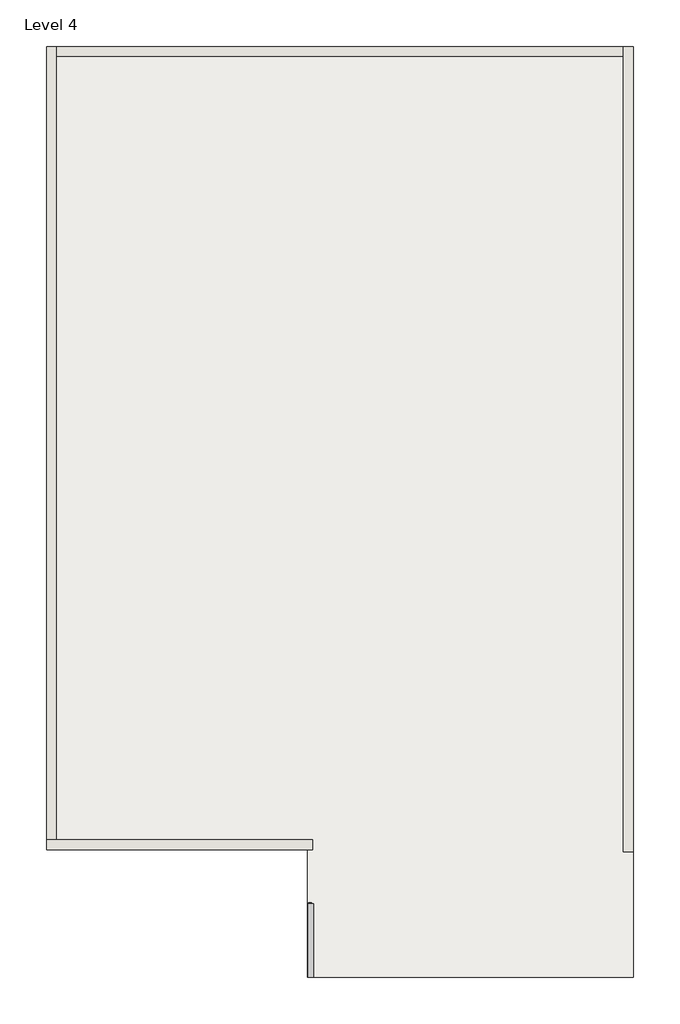
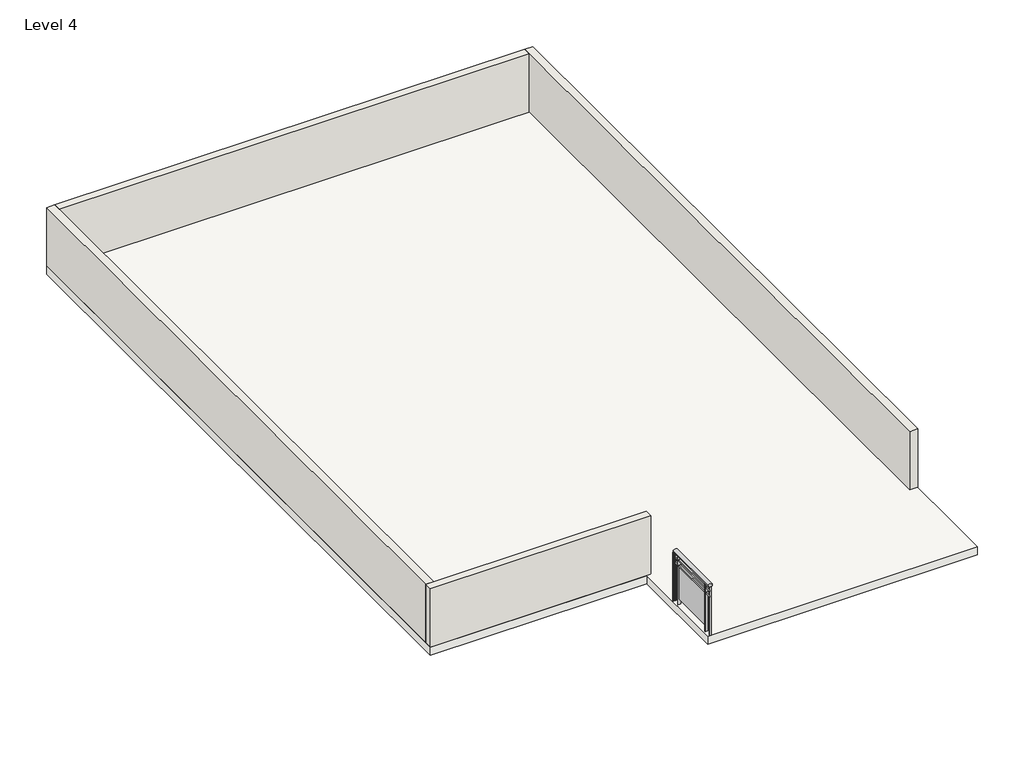
# One storey, incomplete: 4 walls, 1 railing, 1 slab.
"""IFC4 building model written with IfcOpenShell, lengths in millimetres."""

from ifc_helpers import new_model, si_unit, point, frame, origin, place, context, project, spatial, polyline, ellipse_curve, trimmed, outline, extrude, faceted_brep, element, save
from ifc_brep_helpers import plane_surface, extruded_surface, advanced_brep

model = new_model("IFC4")

# Units and contexts
model_context = context("Model", 3, world=origin())
ifc_project = project(units=[si_unit("LENGTHUNIT", "METRE", prefix="MILLI")], contexts=[model_context])

# Site, building, storey
site = spatial("IfcSite", under=ifc_project)
building = spatial("IfcBuilding", under=site)
storey = spatial("IfcBuildingStorey", under=building, Name="Level 4", Elevation=9144.0)

# Railing
placement = place(None, origin())
element("IfcRailing", 1, ObjectType="Glass Panel - Bottom Fill", at=placement, inside=storey, context=model_context, shape_type="SolidModel", body=[
    advanced_brep(
    [(-5042.3449828, -6894.0922127, 10058.4), (-4966.1449828, -6894.0922127, 10058.4), (-5042.3449828, -5842.8058051, 10058.4), (-4966.1449828, -5842.8058051, 10058.4)],
    [
        (0, 1, ellipse_curve(frame((-5004.2449828, -6894.0922127, 10058.4), z_axis=(0.0, -1.0, 0.0), x_axis=(1.0, 0.0, 0.0)), 38.1, 28.575)),
        (1, 0, ellipse_curve(frame((-5004.2449828, -6894.0922127, 10058.4), z_axis=(0.0, -1.0, 0.0), x_axis=(1.0, 0.0, 0.0)), 38.1, 28.575)),
        (2, 3, ellipse_curve(frame((-5004.2449828, -5842.8058051, 10058.4), z_axis=(0.0, 1.0, 0.0), x_axis=(1.0, 0.0, 0.0)), 38.1, 28.575)),
        (3, 2, ellipse_curve(frame((-5004.2449828, -5842.8058051, 10058.4), z_axis=(0.0, 1.0, 0.0), x_axis=(1.0, 0.0, 0.0)), 38.1, 28.575)),
        (0, 2),
        (3, 1),
    ],
    [
        plane_surface(frame((-5004.2449828, -6894.0922127, 10058.4), z_axis=(0.0, -1.0, 0.0), x_axis=(0.0, 0.0, 1.0))),
        plane_surface(frame((-5004.2449828, -5842.8058051, 10058.4), z_axis=(0.0, 1.0, 0.0), x_axis=(0.0, 0.0, 1.0))),
        extruded_surface(trimmed(ellipse_curve(frame((-5004.2449828, -5842.8058051, 10058.4), z_axis=(0.0, -1.0, 0.0), x_axis=(1.0, 0.0, 0.0)), 38.1, 28.575), [point((-5042.3449828, -5842.8058051, 10058.4))], [point((-4966.1449828, -5842.8058051, 10058.4))], True, "CARTESIAN"), (0.0, -1051.2864076000005, 0.0), 1051.2864076000005),
        extruded_surface(trimmed(ellipse_curve(frame((-5004.2449828, -5842.8058051, 10058.4), z_axis=(0.0, -1.0, 0.0), x_axis=(1.0, 0.0, 0.0)), 38.1, 28.575), [point((-4966.1449828, -5842.8058051, 10058.4))], [point((-5042.3449828, -5842.8058051, 10058.4))], True, "CARTESIAN"), (0.0, -1051.2864076000005, 0.0), 1051.2864076000005),
    ],
    [
        (0, [[1, 2]]),
        (1, [[3, 4]]),
        (2, [[-1, 5, -4, 6]]),
        (3, [[-2, -6, -3, -5]]),
    ],
),
    faceted_brep([(-4991.5449828, -6894.0922127, 9969.5), (-5016.9449828, -6894.0922127, 9969.5), (-5016.9449828, -6894.0922127, 9944.1), (-4991.5449828, -6894.0922127, 9944.1), (-4991.5449828, -5830.1058051, 9969.5), (-5016.9449828, -5855.5058051, 9969.5), (-5016.9449828, -5855.5058051, 9944.1), (-4991.5449828, -5830.1058051, 9944.1), (-5039.1884077, -5830.1058051, 9969.5), (-5039.1884077, -5830.1058051, 9944.1), (-5039.1884077, -5855.5058051, 9944.1), (-5039.1884077, -5855.5058051, 9969.5)], [[[0, 1, 2, 3]], [[1, 0, 4, 5]], [[2, 1, 5, 6]], [[3, 2, 6, 7]], [[0, 3, 7, 4]], [[8, 9, 10, 11]], [[5, 4, 8, 11]], [[6, 5, 11, 10]], [[7, 6, 10, 9]], [[4, 7, 9, 8]]]),
    faceted_brep([(-4991.5449828, -6894.0922127, 9867.9), (-5016.9449828, -6894.0922127, 9867.9), (-5016.9449828, -6894.0922127, 9842.5), (-4991.5449828, -6894.0922127, 9842.5), (-4991.5449828, -5830.1058051, 9867.9), (-5016.9449828, -5855.5058051, 9867.9), (-5016.9449828, -5855.5058051, 9842.5), (-4991.5449828, -5830.1058051, 9842.5), (-5039.1884077, -5830.1058051, 9867.9), (-5039.1884077, -5830.1058051, 9842.5), (-5039.1884077, -5855.5058051, 9842.5), (-5039.1884077, -5855.5058051, 9867.9)], [[[0, 1, 2, 3]], [[1, 0, 4, 5]], [[2, 1, 5, 6]], [[3, 2, 6, 7]], [[0, 3, 7, 4]], [[8, 9, 10, 11]], [[5, 4, 8, 11]], [[6, 5, 11, 10]], [[7, 6, 10, 9]], [[4, 7, 9, 8]]]),
    extrude(outline(polyline([(-4978.8449828, -5968.3990089), (-5029.6449828, -5968.3990089), (-5029.6449828, -5955.6990089), (-4978.8449828, -5955.6990089), (-4978.8449828, -5968.3990089)])), frame((0.0, 0.0, 9144.0), z_axis=(0.0, 0.0, 1.0), x_axis=(1.0, 0.0, 0.0)), (0.0, 0.0, 1.0), 885.825),
    extrude(outline(polyline([(-5010.7801398, -6774.8490089), (-5010.7801398, -5962.0490089), (-5004.4301398, -5962.0490089), (-5004.4301398, -6774.8490089), (-5010.7801398, -6774.8490089)])), frame((0.0, 0.0, 9245.6), z_axis=(0.0, 0.0, 1.0), x_axis=(1.0, 0.0, 0.0)), (0.0, 0.0, 1.0), 596.9),
    extrude(outline(polyline([(-4978.8449828, -6781.1990089), (-5029.6449828, -6781.1990089), (-5029.6449828, -6768.4990089), (-4978.8449828, -6768.4990089), (-4978.8449828, -6781.1990089)])), frame((0.0, 0.0, 9144.0), z_axis=(0.0, 0.0, 1.0), x_axis=(1.0, 0.0, 0.0)), (0.0, 0.0, 1.0), 885.825),
    extrude(outline(polyline([(-4994.7199828, -5852.3308051), (-5013.7699828, -5852.3308051), (-5013.7699828, -5833.2808051), (-4994.7199828, -5833.2808051), (-4994.7199828, -5852.3308051)])), frame((0.0, 0.0, 9144.0), z_axis=(0.0, 0.0, 1.0), x_axis=(1.0, 0.0, 0.0)), (0.0, 0.0, 1.0), 885.825),
    extrude(outline(polyline([(-5026.4884077, -5833.2808051), (-5026.4884077, -5852.3308051), (-5045.5384077, -5852.3308051), (-5045.5384077, -5833.2808051), (-5026.4884077, -5833.2808051)])), frame((0.0, 0.0, 9144.0), z_axis=(0.0, 0.0, 1.0), x_axis=(1.0, 0.0, 0.0)), (0.0, 0.0, 1.0), 885.825),
    extrude(outline(polyline([(-4994.7199828, -6900.4422127), (-5013.7699828, -6900.4422127), (-5013.7699828, -6881.3922127), (-4994.7199828, -6881.3922127), (-4994.7199828, -6900.4422127)])), frame((0.0, 0.0, 9144.0), z_axis=(0.0, 0.0, 1.0), x_axis=(1.0, 0.0, 0.0)), (0.0, 0.0, 1.0), 885.825),
])

# Slab
element("IfcSlab", 2, ObjectType="6\"", at=placement, inside=storey, context=model_context, shape_type="SweptSolid", body=[
    extrude(outline(polyline([(-375.7785282, 6451.8796337), (-375.7785282, -6894.0922127), (-5049.0296925, -6894.0922127), (-5049.0296925, -5067.0203663), (-8797.003757, -5067.0203663), (-8797.003757, 6451.8796337), (-375.7785282, 6451.8796337)])), frame((0.0, 0.0, 8991.6), z_axis=(0.0, 0.0, 1.0), x_axis=(1.0, 0.0, 0.0)), (0.0, 0.0, 1.0), 152.4),
])

# Walls
element("IfcWall", 3, ObjectType="4.5\"", at=placement, inside=storey, context=model_context, shape_type="Brep", body=[
    faceted_brep([(-515.4785282, 6451.8796337, 9144.0), (-515.4785282, 6312.1796337, 9144.0), (-515.4785282, -5098.7703663, 9144.0), (-515.4785282, -5098.7703663, 10210.8), (-515.4785282, 6312.1796337, 10210.8), (-515.4785282, 6451.8796337, 10210.8), (-375.7785282, 6451.8796337, 9144.0), (-375.7785282, 6451.8796337, 10210.8), (-375.7785282, -5098.7703663, 10210.8), (-375.7785282, -5098.7703663, 9144.0)], [[[0, 1, 2, 3, 4, 5]], [[6, 7, 8, 9]], [[2, 1, 0, 6, 9]], [[3, 2, 9, 8]], [[5, 4, 3, 8, 7]], [[0, 5, 7, 6]]]),
])
element("IfcWall", 4, ObjectType="4.5\"", at=placement, inside=storey, context=model_context, shape_type="Brep", body=[
    faceted_brep([(-4979.1796925, -4927.3203663, 9144.0), (-8657.303757, -4927.3203663, 9144.0), (-8797.003757, -4927.3203663, 9144.0), (-8797.003757, -4927.3203663, 10210.8), (-8657.303757, -4927.3203663, 10210.8), (-4979.1796925, -4927.3203663, 10210.8), (-4979.1796925, -5067.0203663, 9144.0), (-4979.1796925, -5067.0203663, 10210.8), (-8797.003757, -5067.0203663, 10210.8), (-8797.003757, -5067.0203663, 9144.0)], [[[0, 1, 2, 3, 4, 5]], [[6, 7, 8, 9]], [[2, 1, 0, 6, 9]], [[5, 4, 3, 8, 7]], [[0, 5, 7, 6]], [[3, 2, 9, 8]]]),
])
element("IfcWall", 5, ObjectType="4.5\"", at=placement, inside=storey, context=model_context, shape_type="Brep", body=[
    faceted_brep([(-8657.303757, -4927.3203663, 9144.0), (-8657.303757, 6312.1796337, 9144.0), (-8657.303757, 6451.8796337, 9144.0), (-8657.303757, 6451.8796337, 10210.8), (-8657.303757, 6312.1796337, 10210.8), (-8657.303757, -4927.3203663, 10210.8), (-8797.003757, -4927.3203663, 9144.0), (-8797.003757, -4927.3203663, 10210.8), (-8797.003757, 6451.8796337, 10210.8), (-8797.003757, 6451.8796337, 9144.0)], [[[0, 1, 2, 3, 4, 5]], [[6, 7, 8, 9]], [[2, 1, 0, 6, 9]], [[5, 4, 3, 8, 7]], [[0, 5, 7, 6]], [[3, 2, 9, 8]]]),
])
element("IfcWall", 6, ObjectType="4.5\"", at=placement, inside=storey, context=model_context, shape_type="SweptSolid", body=[
    extrude(outline(polyline([(-515.4785282, 6312.1796337), (-8657.303757, 6312.1796337), (-8657.303757, 6451.8796337), (-515.4785282, 6451.8796337), (-515.4785282, 6312.1796337)])), frame((0.0, 0.0, 9144.0), z_axis=(0.0, 0.0, 1.0), x_axis=(1.0, 0.0, 0.0)), (0.0, 0.0, 1.0), 1066.8),
])

save(model, "model.ifc")

# Revit data of these elements
# Type "Glass Panel - Bottom Fill"
#   Assembly Code = "C2010400"
#   built-in parameter 1008612 = 0.0416667 (stored number, unit not read)
#   built-in parameter 1008611 = 0.0416667 (stored number, unit not read)
#   built-in parameter 1008609 = 0.333333 (stored number, unit not read)
#   built-in parameter 1008604 = 0.166667 (stored number, unit not read)
#   built-in parameter 1008603 = 0.166667 (stored number, unit not read)
#   Railing Height = 36"
#   built-in parameter 1008630 = 2
#   built-in parameter 1008610 = 2
#   built-in parameter 1008618 = Baluster - Square : 3/4"
# Type "6\""
#   Assembly Code = "B1010"
#   Function = 0
#   Layers, outside or top first: 6" no material (function 1)
# Type "4.5\""
#   Assembly Code = "B2010"
#   Layers, outside or top first: 0.5" "INNER WALL" (function 1); 4.5" "BRICK MATERIAL" (function 1); 0.5" "INNER WALL" (function 1)
# Element 1 (IfcRailing, "Glass Panel - Bottom Fill")
#   Phase Created = New Construction
#   Materials on its faces: "Glass"
# Element 2 (IfcSlab, "6\"")
#   Height Offset From Level = 0"
#   Phase Created = New Construction
#   Materials on its faces: "Default Floor"
# Elements 3, 4, 5 (IfcWall, "4.5\"")
#   Top Offset = 0"
#   Base Offset = 0"
#   Unconnected Height = 42"
#   wall height = 42"
#   Phase Created = New Construction
#   Base Constraint = Level 4
#   Materials on its faces: "INNER WALL", "Default Wall"
# Element 6 (IfcWall, "4.5\"")
#   Top Offset = 0"
#   Base Offset = 0"
#   Unconnected Height = 42"
#   wall height = 42"
#   Phase Created = New Construction
#   Base Constraint = Level 4
#   Materials on its faces: "Default Wall", "INNER WALL"
# Materials
#   "INNER WALL": class "Generic", colour RGB 112 107 80, transparency 0, Cost = 0
#   "BRICK MATERIAL": class "Generic", colour RGB 86 33 38, transparency 0, Cost = 0
#   "Glass": class "Glass", colour RGB 0 128 192, transparency 0.75, Description = "Soda Lime Glass", Cost = 0
#   "Default Floor": colour RGB 128 128 128, transparency 0, Cost = 0
#   "Default Wall": colour RGB 128 128 128, transparency 0, Cost = 0
